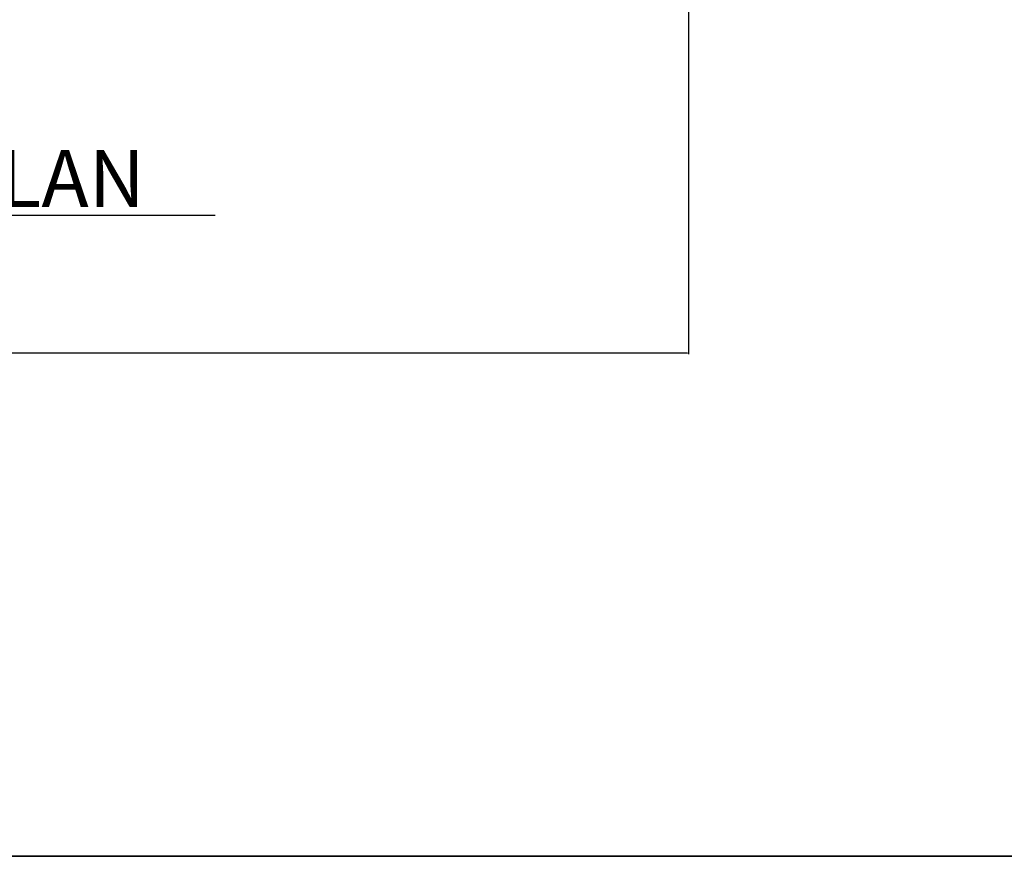
# Model space of a CAD drawing. Units: inches. Extents: x 1441 to 2460, y 1648 to 2683.
# Tile 2 of 35: x 1760 to 1950, y 1648 to 1810. Entities that reach past the tile are written whole.
import ezdxf

# ---------------------------------------------------------------- set-up
doc = ezdxf.new("R2010")
doc.units = ezdxf.units.IN
for name, color, linetype, lineweight in [('A-ANNO-DIMS', 2, 'Continuous', 18), ('A-ANNO-TITL', 7, 'Continuous', 30), ('A-ANNO-TTLB', 7, 'Continuous', 35)]:
    doc.layers.add(name, color=color, linetype=linetype, lineweight=lineweight)
doc.styles.get("Standard").update_dxf_attribs({"font": 'arial.ttf'})
doc.dimstyles.get("Standard").update_dxf_attribs({"dimtxt": 0.18, "dimasz": 0.18, "dimexe": 0.18, "dimexo": 0.0625, "dimgap": 0.09, "dimtad": 0, "dimtih": 1, "dimtoh": 1, "dimdec": 4, "dimzin": 0, "dimdsep": 46, "dimtxsty": 'Standard', "dimcen": 0.09, "dimadec": 0, "dimazin": 0, "dimtfac": 1, "dimtdec": 4, "dimtofl": 0, "dimtmove": 0, "dimatfit": 3, "dimfxl": 1, "dimtolj": 1, "dimtzin": 0, "dimarcsym": 0})

# ---------------------------------------------------------------- blocks, each defined once
blk = doc.blocks.new('*D66')
at = {"layer": 'A-ANNO-DIMS', "color": 0, "lineweight": -2, "transparency": 16777216}
for p, q in [((1568.89, 1834.13), (1568.89, 1745.01)), ((1889.39, 1834.13), (1889.39, 1745.01)), ((1569.07, 1745.19), (1728.74, 1745.19)), ((1889.21, 1745.19), (1729.53, 1745.19))]:
    blk.add_line(p, q, dxfattribs=at)
at = {"layer": 'A-ANNO-DIMS', "color": 0, "transparency": 16777216}
for points in [[(1569.07, 1745.22), (1569.07, 1745.16), (1568.89, 1745.19)], [(1889.21, 1745.22), (1889.21, 1745.16), (1889.39, 1745.19)]]:
    blk.add_solid(points, dxfattribs=at)
at = {"layer": 'Defpoints', "color": 0, "transparency": 16777216}
for p in [(1568.89, 1834.2), (1889.39, 1834.2), (1889.39, 1745.19)]:
    blk.add_point(p, dxfattribs=at)
at = {"layer": 'A-ANNO-DIMS', "color": 0, "transparency": 16777216, "insert": (1729.14, 1745.19), "char_height": 0.18, "attachment_point": 5}
blk.add_mtext('\\A1;320.5', dxfattribs=at)

msp = doc.modelspace()

# ---------------------------------------------------------------- linework, layer by layer
at = {"layer": 'A-ANNO-TITL'}
msp.add_line((1629.5852, 1771.8364), (1798.1081, 1771.8364), dxfattribs=at)
at = {"layer": 'A-ANNO-TTLB'}
msp.add_lwpolyline([(1440.5107, 2682.6413), (2460.193, 2682.6413), (2460.193, 1648.08), (1440.5107, 1648.08)], close=True, dxfattribs=at)

# ---------------------------------------------------------------- texts
at = {"layer": 'A-ANNO-TITL', "insert": (1628.9764, 1784.3785), "char_height": 11, "attachment_point": 1}
msp.add_mtext_dynamic_manual_height_columns('GROUND FLOOR PLAN', width=244.599836, gutter_width=12.5, heights=[0], dxfattribs=at)

# ---------------------------------------------------------------- dimensions: what is measured, and where the dimension line sits
at = {"layer": 'A-ANNO-DIMS'}
dim = msp.add_linear_dim(base=(1889.3859, 1745.1864), p1=(1568.8859, 1834.1952), p2=(1889.3859, 1834.1952), dimstyle='Standard', override={"dimdec": 1, "dimlfac": 1, "dimrnd": 0, "dimzin": 0, "dimdsep": 46, "dimlunit": 2}, dxfattribs=at)
dim.commit()
dim.dimension.update_dxf_attribs({"geometry": '*D66', "text_midpoint": (1729.1359, 1745.1864)})

doc.saveas('drawing.dxf')
